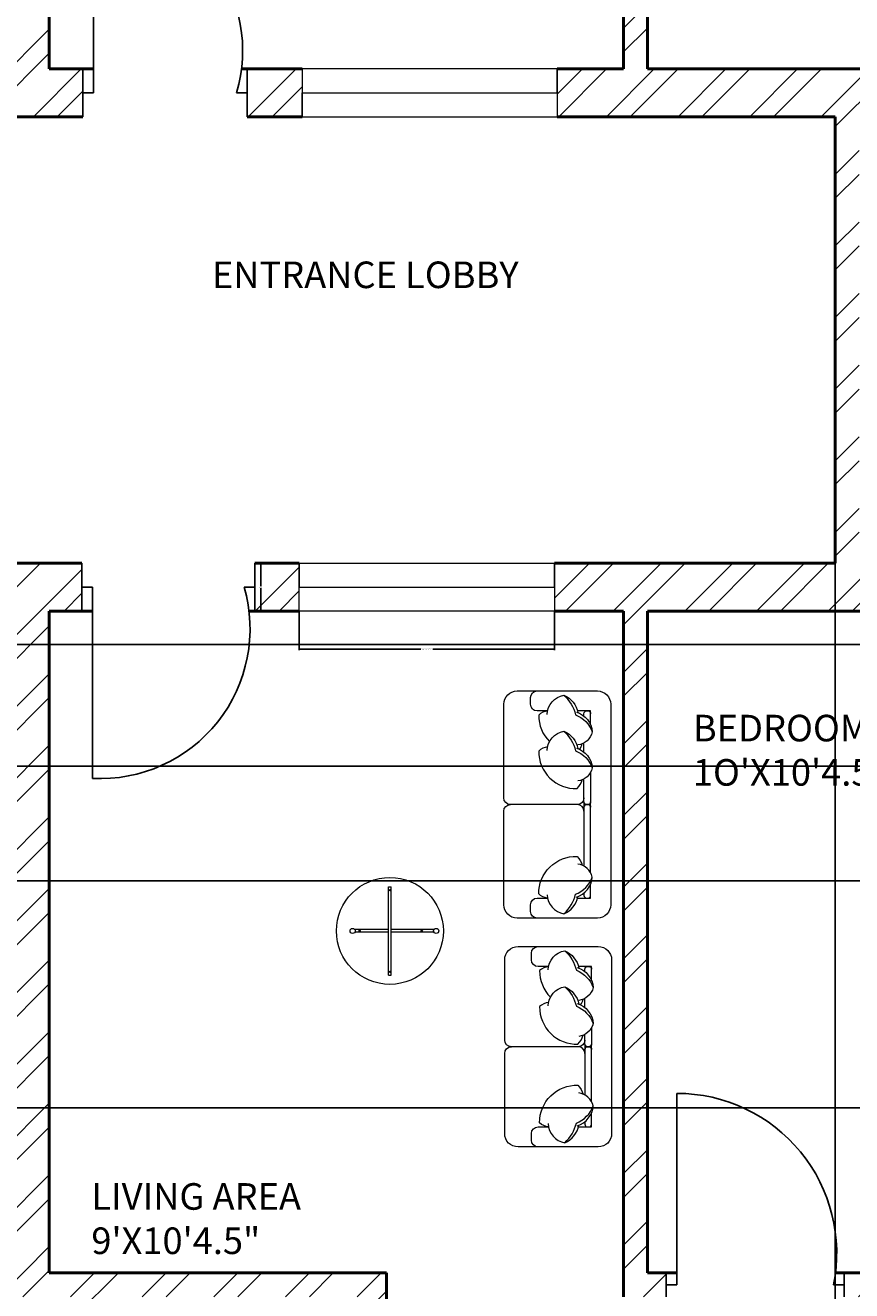
# Model space of a CAD drawing. Units: inches. Extents: x 1980 to 2738, y 1471 to 2568.
# Tile 14 of 22: x 2363 to 2519, y 1874 to 2112. Entities that reach past the tile are written whole.
import ezdxf

# ---------------------------------------------------------------- set-up
doc = ezdxf.new("R2010")
doc.units = ezdxf.units.IN
for name, color, linetype, lineweight in [('A-ANNO-DIMS', 2, 'Continuous', 18), ('A-AREA-IDEN', 7, 'Continuous', 18), ('A-DOOR', 31, 'Continuous', 25), ('A-FURN', 8, 'Continuous', 18), ('A-GLAZ', 141, 'Continuous', 18), ('A-WALL', 7, 'Continuous', 50)]:
    doc.layers.add(name, color=color, linetype=linetype, lineweight=lineweight)
doc.layers.add('A-WALL-PATT', color=9, linetype='Continuous', lineweight=13, true_color=0xd19cc7)
doc.styles.get("Standard").update_dxf_attribs({"font": 'arial.ttf'})
doc.dimstyles.get("Standard").update_dxf_attribs({"dimtxt": 0.18, "dimasz": 0.18, "dimexe": 0.18, "dimexo": 0.0625, "dimgap": 0.09, "dimtad": 0, "dimtih": 1, "dimtoh": 1, "dimdec": 4, "dimzin": 0, "dimdsep": 46, "dimtxsty": 'Standard', "dimcen": 0.09, "dimadec": 0, "dimazin": 0, "dimtfac": 1, "dimtdec": 4, "dimtofl": 0, "dimtmove": 0, "dimatfit": 3, "dimfxl": 1, "dimtolj": 1, "dimtzin": 0, "dimarcsym": 0})

# ---------------------------------------------------------------- blocks, each defined once
blk = doc.blocks.new('table r 343')
at = {"color": 0}
for p, q in [((-10, 10), (-10, 262.1)), ((10, 10), (10, 262.1)), ((-330.3, 10), (330.3, 10)), ((-330.3, 10), (-330.3, -10)), ((330.3, 10), (330.3, -10)), ((-330.3, -10), (330.3, -10)), ((-10, -330.3), (-10, -10)), ((10, -330.3), (10, -10))]:
    blk.add_line(p, q, dxfattribs=at)
for centre, radius in [((0, 0), 400), ((0, 278.7), 19.4), ((0, 226.8), 5), ((-306.1, 0), 5), ((306.1, 0), 5), ((0, -238.1), 5), ((0, -346.9), 19.4)]:
    blk.add_circle(centre, radius, dxfattribs=at)
blk = doc.blocks.new('WIN-48IN-WALL')
for p, q in [((0, 4.5), (0, 9)), ((0, 9), (0, 0)), ((48, 9), (0, 9)), ((48, 0), (48, 9)), ((48, 9), (48, 4.5)), ((48, 4.5), (0, 4.5)), ((0, 0), (48, 0))]:
    blk.add_line(p, q)
blk = doc.blocks.new('*D33')
at = {"layer": 'A-ANNO-DIMS', "color": 0, "lineweight": -2, "transparency": 16777216}
for p, q in [((2414.6, 2002.14), (2414.6, 1994.83)), ((2462.6, 2002.14), (2462.6, 1994.83)), ((2414.78, 1995.01), (2437.48, 1995.01)), ((2462.42, 1995.01), (2439.71, 1995.01))]:
    blk.add_line(p, q, dxfattribs=at)
at = {"layer": 'A-ANNO-DIMS', "color": 0, "transparency": 16777216}
for points in [[(2414.78, 1995.04), (2414.78, 1994.98), (2414.6, 1995.01)], [(2462.42, 1995.04), (2462.42, 1994.98), (2462.6, 1995.01)]]:
    blk.add_solid(points, dxfattribs=at)
at = {"layer": 'Defpoints', "color": 0, "transparency": 16777216}
for p in [(2414.6, 2002.21), (2462.6, 2002.21), (2414.6, 1995.01)]:
    blk.add_point(p, dxfattribs=at)
at = {"layer": 'A-ANNO-DIMS', "color": 0, "transparency": 16777216, "insert": (2438.6, 1995.01), "char_height": 0.18, "attachment_point": 5}
blk.add_mtext('\\A1;WINDOW 48 TYP.', dxfattribs=at)
blk = doc.blocks.new('*D34')
at = {"layer": 'A-ANNO-DIMS', "color": 0, "lineweight": -2, "transparency": 16777216}
for p, q in [((2414.53, 2011.21), (2407.22, 2011.21)), ((2407.4, 2011.03), (2407.4, 2006.89)), ((2407.4, 2002.39), (2407.4, 2006.52)), ((2414.53, 2002.21), (2407.22, 2002.21))]:
    blk.add_line(p, q, dxfattribs=at)
at = {"layer": 'A-ANNO-DIMS', "color": 0, "transparency": 16777216}
for points in [[(2407.37, 2011.03), (2407.43, 2011.03), (2407.4, 2011.21)], [(2407.37, 2002.39), (2407.43, 2002.39), (2407.4, 2002.21)]]:
    blk.add_solid(points, dxfattribs=at)
at = {"layer": 'Defpoints', "color": 0, "transparency": 16777216}
for p in [(2407.4, 2011.21), (2414.6, 2011.21), (2414.6, 2002.21)]:
    blk.add_point(p, dxfattribs=at)
at = {"layer": 'A-ANNO-DIMS', "color": 0, "transparency": 16777216, "insert": (2407.4, 2006.71), "char_height": 0.18, "attachment_point": 5}
blk.add_mtext('\\A1;9 TYP.', dxfattribs=at)
blk = doc.blocks.new('*D41')
at = {"layer": 'A-ANNO-DIMS', "color": 0, "lineweight": -2, "transparency": 16777216}
for p, q in [((2298.65, 2095.14), (2298.65, 1533.71)), ((2515.4, 2095.14), (2515.4, 1533.71)), ((2298.83, 1533.89), (2406.56, 1533.89)), ((2515.22, 1533.89), (2407.49, 1533.89))]:
    blk.add_line(p, q, dxfattribs=at)
at = {"layer": 'A-ANNO-DIMS', "color": 0, "transparency": 16777216}
for points in [[(2298.83, 1533.92), (2298.83, 1533.86), (2298.65, 1533.89)], [(2515.22, 1533.92), (2515.22, 1533.86), (2515.4, 1533.89)]]:
    blk.add_solid(points, dxfattribs=at)
at = {"layer": 'Defpoints', "color": 0, "transparency": 16777216}
for p in [(2298.65, 2095.21), (2515.4, 2095.21), (2515.4, 1533.89)]:
    blk.add_point(p, dxfattribs=at)
at = {"layer": 'A-ANNO-DIMS', "color": 0, "transparency": 16777216, "insert": (2407.03, 1533.89), "char_height": 0.18, "attachment_point": 5}
blk.add_mtext('\\A1;216.75', dxfattribs=at)
blk = doc.blocks.new('*D55')
at = {"layer": 'A-ANNO-DIMS', "color": 0, "lineweight": -2, "transparency": 16777216}
for p, q in [((2269.76, 1951.46), (2689.91, 1951.46)), ((2689.73, 1951.28), (2689.73, 1930.28)), ((2689.73, 1908.91), (2689.73, 1929.91)), ((2269.76, 1908.73), (2689.91, 1908.73))]:
    blk.add_line(p, q, dxfattribs=at)
at = {"layer": 'A-ANNO-DIMS', "color": 0, "transparency": 16777216}
for points in [[(2689.7, 1951.28), (2689.76, 1951.28), (2689.73, 1951.46)], [(2689.7, 1908.91), (2689.76, 1908.91), (2689.73, 1908.73)]]:
    blk.add_solid(points, dxfattribs=at)
at = {"layer": 'Defpoints', "color": 0, "transparency": 16777216}
for p in [(2269.7, 1951.46), (2689.73, 1951.46), (2269.7, 1908.73)]:
    blk.add_point(p, dxfattribs=at)
at = {"layer": 'A-ANNO-DIMS', "color": 0, "transparency": 16777216, "insert": (2689.73, 1930.09), "char_height": 0.18, "attachment_point": 5}
blk.add_mtext('\\A1;42.735', dxfattribs=at)
blk = doc.blocks.new('*D56')
at = {"layer": 'A-ANNO-DIMS', "color": 0, "lineweight": -2, "transparency": 16777216}
for p, q in [((2114.15, 1995.93), (2689.91, 1995.93)), ((2689.73, 1995.75), (2689.73, 1984.65)), ((2689.73, 1973.18), (2689.73, 1984.28)), ((2114.15, 1973), (2689.91, 1973))]:
    blk.add_line(p, q, dxfattribs=at)
at = {"layer": 'A-ANNO-DIMS', "color": 0, "transparency": 16777216}
for points in [[(2689.7, 1995.75), (2689.76, 1995.75), (2689.73, 1995.93)], [(2689.7, 1973.18), (2689.76, 1973.18), (2689.73, 1973)]]:
    blk.add_solid(points, dxfattribs=at)
at = {"layer": 'Defpoints', "color": 0, "transparency": 16777216}
for p in [(2114.08, 1995.93), (2689.73, 1995.93), (2114.08, 1973)]:
    blk.add_point(p, dxfattribs=at)
at = {"layer": 'A-ANNO-DIMS', "color": 0, "transparency": 16777216, "insert": (2689.73, 1984.47), "char_height": 0.18, "attachment_point": 5}
blk.add_mtext('\\A1;22.935', dxfattribs=at)

msp = doc.modelspace()

# ---------------------------------------------------------------- hatches: boundary and pattern name
at = {"layer": 'A-WALL-PATT'}
h = msp.add_hatch(dxfattribs=at)
h.set_pattern_fill('ANSI32', color=256)
h.paths.add_polyline_path([(2257.5661, 2416.2064), (2257.5661, 2420.7064), (2250.5833, 2420.7064), (2250.5833, 2462.7064), (2246.0833, 2462.7064), (2246.0833, 2420.7064), (2237.0791, 2420.7064), (2237.0791, 2411.7064), (2246.0833, 2411.7064), (2246.0833, 2291.7064), (2242.6109, 2291.7064), (2242.6109, 2287.2064), (2246.0833, 2287.2064), (2250.5833, 2287.2064), (2250.5833, 2291.7064), (2250.5833, 2411.7064), (2257.5661, 2411.7064)])
h.paths.add_polyline_path([(2387.0396, 2416.2064), (2387.0396, 2420.7064), (2367.5833, 2420.7064), (2367.5833, 2462.7064), (2358.5833, 2462.7064), (2358.5833, 2420.7064), (2329.3087, 2420.7064), (2329.3087, 2411.7064), (2358.5833, 2411.7064), (2358.5833, 2321.7275), (2358.5833, 2309.7064), (2347.3089, 2309.7064), (2293.3089, 2309.7064), (2293.3089, 2259.0771), (2297.8089, 2259.0771), (2297.8089, 2305.2064), (2347.3089, 2305.2064), (2347.3089, 2284.7412), (2351.8089, 2284.7412), (2351.8089, 2305.2064), (2372.3188, 2305.2064), (2372.3761, 2284.3899), (2377.0295, 2284.3899), (2377.0295, 2299.3058), (2377.0295, 2305.2064), (2426.5295, 2305.2064), (2426.5295, 2257.5573), (2431.0295, 2257.5573), (2431.0295, 2309.7064), (2377.0295, 2309.7064), (2367.5833, 2309.7064), (2367.5833, 2321.7275), (2367.5833, 2411.7064), (2387.0396, 2411.7064)])
h.paths.add_polyline_path([(2448.5267, 2416.2064), (2448.5267, 2420.7064), (2423.0396, 2420.7064), (2423.0396, 2411.7064), (2448.5267, 2411.7064)])
h.paths.add_polyline_path([(2130.9128, 2416.2064), (2130.9128, 2420.7064), (2105.0833, 2420.7064), (2105.0833, 2386.6942), (2114.0833, 2386.6942), (2114.0833, 2411.7064), (2130.9128, 2411.7064)])
h.paths.add_polyline_path([(2212.9478, 2420.7064), (2190.9128, 2420.7064), (2190.9128, 2411.7064), (2212.9478, 2411.7064), (2212.9478, 2416.2064)])
h.paths.add_polyline_path([(2114.0833, 2326.6942), (2105.0833, 2326.6942), (2105.0833, 2291.7064), (2081.0833, 2291.7064), (2081.0833, 2287.2064), (2105.0833, 2287.2064), (2105.0833, 2276.1935), (2114.0833, 2276.1935), (2114.0833, 2287.2064), (2166.3825, 2287.2064), (2166.3825, 2289.4564), (2166.3825, 2291.7064), (2114.0833, 2291.7064)])
h.paths.add_polyline_path([(2114.0833, 2252.1935), (2105.0833, 2252.1935), (2105.0833, 2233.2064), (2081.0833, 2233.2064), (2081.0833, 2228.7064), (2105.0833, 2228.7064), (2105.0833, 2213.4478), (2114.0833, 2213.4478), (2114.0833, 2228.7064), (2195.0833, 2228.7064), (2199.5833, 2228.7064), (2208.4455, 2228.7064), (2208.4455, 2230.9564), (2208.4455, 2233.2064), (2199.5833, 2233.2064), (2199.5833, 2287.2064), (2206.8904, 2287.2064), (2206.8904, 2289.4564), (2206.8904, 2291.7064), (2189.446, 2291.7064), (2189.446, 2289.4564), (2189.446, 2287.2064), (2195.0833, 2287.2064), (2195.0833, 2233.2064), (2114.0833, 2233.2064)])
h.paths.add_polyline_path([(2114.0833, 2153.4478), (2109.5833, 2153.4478), (2105.0833, 2153.4478), (2105.0833, 2135.2374), (2114.0833, 2135.2374)], flags=17)
h.paths.add_polyline_path([(2135.9619, 2095.4081), (2140.1805, 2095.4081), (2140.1805, 2104.2064), (2114.0833, 2104.2064), (2114.0833, 2110.3997), (2109.5833, 2110.3997), (2105.0833, 2110.3997), (2105.0833, 2104.2064), (2081.0833, 2104.2064), (2081.0833, 2099.7064), (2105.0833, 2099.7064), (2127.5416, 2099.8532), (2127.5416, 2056.9393), (2136.2133, 2056.9393)], flags=17)
h.paths.add_polyline_path([(2255.4895, 2104.2064), (2250.5833, 2104.2064), (2250.5833, 2233.2064), (2246.0833, 2233.2064), (2242.4941, 2233.2064), (2242.4941, 2228.7064), (2246.0833, 2228.7064), (2246.0833, 2104.2064), (2163.6825, 2104.2064), (2163.6825, 2099.8072), (2163.6825, 2095.4081), (2191.4325, 2095.4081), (2191.4325, 2011.2064), (2186.0833, 2011.2064), (2136.5143, 2010.8824), (2136.3702, 2032.9403), (2131.9559, 2032.9115), (2127.5416, 2032.8826), (2127.5416, 2006.7064), (2105.0833, 2006.7064), (2081.0833, 2006.7064), (2081.0833, 2002.2064), (2105.0833, 2002.2064), (2105.0833, 1995.9329), (2114.0833, 1995.9329), (2114.0833, 2002.2064), (2246.0833, 2002.2064), (2246.0833, 1877.7064), (2242.1358, 1877.7064), (2242.1358, 1873.2064), (2250.5833, 1873.2064), (2250.5833, 2002.2064), (2255.3335, 2002.2064), (2255.3335, 2011.2064), (2195.9325, 2011.2064), (2195.9325, 2095.2064), (2255.4895, 2095.2064), (2255.4895, 2099.5471)])
h.paths.add_polyline_path([(2199.5833, 1873.2064), (2209.827, 1873.2064), (2209.827, 1875.4564), (2209.827, 1877.7064), (2114.0833, 1877.7064), (2114.0833, 1890.0968), (2105.0833, 1890.0968), (2105.0833, 1877.7064), (2081.0833, 1877.7064), (2081.0833, 1873.2064), (2105.0833, 1873.2064), (2105.0833, 1857.7279), (2114.0833, 1857.7279), (2114.0833, 1873.2064), (2195.0833, 1873.2064), (2195.0833, 1819.2064), (2190.298, 1819.2064), (2190.298, 1814.7064), (2209.8976, 1814.7064), (2209.8976, 1816.9564), (2209.8976, 1819.2064), (2199.5833, 1819.2064)])
h.paths.add_polyline_path([(2114.0833, 1814.7064), (2166.2538, 1814.7064), (2166.2538, 1816.9564), (2166.2538, 1819.2064), (2114.0833, 1819.2064), (2114.0833, 1833.7279), (2109.5833, 1833.7279), (2105.0833, 1833.7279), (2105.0833, 1819.2064), (2081.0833, 1819.2064), (2081.0833, 1814.7064), (2105.0833, 1814.7064), (2105.0833, 1782.5516), (2114.0833, 1782.5516)])
h.paths.add_polyline_path([(2114.0833, 1722.5516), (2109.5833, 1722.5516), (2105.0833, 1722.5516), (2105.0833, 1685.7064), (2124.5104, 1685.7064), (2124.5104, 1690.2064), (2124.5104, 1694.7064), (2114.0833, 1694.7064)])
h.paths.add_polyline_path([(2218.8787, 1694.7064), (2184.5104, 1694.7064), (2184.5104, 1685.7064), (2218.8787, 1685.7064), (2218.8787, 1690.2064)])
h.paths.add_polyline_path([(2250.5833, 1819.2064), (2242.6431, 1819.2064), (2242.6431, 1816.9564), (2242.6431, 1814.7064), (2246.0833, 1814.7064), (2246.0833, 1694.7064), (2240.4035, 1694.7064), (2240.4035, 1690.2064), (2240.4035, 1685.7064), (2246.0833, 1685.7064), (2246.0833, 1643.7064), (2250.5833, 1643.7064), (2250.5833, 1685.7064), (2255.9859, 1685.7064), (2255.9859, 1690.2064), (2255.9859, 1694.7064), (2250.5833, 1694.7064)])
h.paths.add_polyline_path([(2297.4764, 1694.7064), (2279.3934, 1694.7064), (2279.3934, 1690.2064), (2279.3934, 1685.7064), (2297.4764, 1685.7064), (2297.4764, 1690.2064)])
h.paths.add_polyline_path([(2377.1596, 1694.7064), (2367.5833, 1694.7064), (2367.5833, 1787.7064), (2431.0295, 1787.7064), (2431.0295, 1792.2064), (2431.0295, 1849.4149), (2428.7795, 1849.4149), (2426.5295, 1849.4149), (2426.5295, 1792.2064), (2421.5833, 1792.2064), (2367.5833, 1792.2064), (2297.8089, 1792.2064), (2297.8089, 1850.2946), (2295.5589, 1850.2946), (2293.3089, 1850.2946), (2293.3089, 1792.2064), (2293.3089, 1787.7064), (2297.8089, 1787.7064), (2358.5833, 1787.7064), (2358.5833, 1694.7064), (2333.4764, 1694.7064), (2333.4764, 1685.7064), (2358.5833, 1685.7064), (2358.5833, 1643.7064), (2367.5833, 1643.7064), (2367.5833, 1685.7064), (2377.1596, 1685.7064)])
h.paths.add_polyline_path([(2442.4912, 1694.7064), (2413.1596, 1694.7064), (2413.1596, 1685.7064), (2442.4912, 1685.7064)])
h.paths.add_polyline_path([(2480.0833, 1814.7064), (2483.4816, 1814.7064), (2483.4816, 1817.9384), (2483.4816, 1819.2064), (2475.5833, 1819.2064), (2475.5833, 1694.7064), (2470.7283, 1694.7064), (2470.7283, 1685.7064), (2475.5833, 1685.7064), (2475.5833, 1643.7064), (2480.0833, 1643.7064), (2480.0833, 1685.7064), (2486.3293, 1685.7064), (2486.3293, 1690.2064), (2486.3293, 1694.7064), (2480.0833, 1694.7064)])
h.paths.add_polyline_path([(2621.0833, 1721.7349), (2612.0833, 1721.7349), (2612.0833, 1694.7064), (2586.1453, 1694.7064), (2586.1453, 1685.7064), (2621.0833, 1685.7064)])
h.paths.add_polyline_path([(2526.1453, 1690.2064), (2526.1453, 1694.7064), (2511.584, 1694.7064), (2511.584, 1690.2064), (2511.584, 1685.7064), (2526.1453, 1685.7064)])
h.paths.add_polyline_path([(2645.0833, 1819.2064), (2621.0833, 1819.2064), (2621.0833, 1835.8527), (2616.5833, 1835.8527), (2612.0833, 1835.8527), (2612.0833, 1819.2064), (2560.2541, 1819.2064), (2560.2541, 1814.7064), (2612.0833, 1814.7064), (2612.0833, 1781.7349), (2621.0833, 1781.7349), (2621.0833, 1814.7064), (2645.0833, 1814.7064)])
h.paths.add_polyline_path([(2645.0833, 1877.7064), (2621.0833, 1877.7064), (2621.0833, 1886.4375), (2612.0833, 1886.4375), (2612.0833, 1877.7064), (2517.1032, 1877.7064), (2517.1032, 1875.4564), (2517.1032, 1873.2064), (2526.5833, 1873.2064), (2526.5833, 1819.2064), (2516.6454, 1819.2064), (2516.6454, 1816.9564), (2516.6454, 1814.7064), (2536.4445, 1814.7064), (2536.4445, 1816.9564), (2536.4445, 1819.2064), (2531.0833, 1819.2064), (2531.0833, 1873.2064), (2612.0833, 1873.2064), (2612.0833, 1859.8527), (2621.0833, 1859.8527), (2621.0833, 1873.2064), (2645.0833, 1873.2064)])
h.paths.add_polyline_path([(2645.0833, 2006.7064), (2621.0833, 2006.7064), (2588.5085, 2006.7064), (2588.5085, 2052.9125), (2579.9045, 2052.9125), (2579.9045, 2011.2064), (2519.9045, 2011.2064), (2519.9045, 2095.2064), (2553.1204, 2095.2064), (2553.1204, 2104.2064), (2480.0833, 2104.2064), (2480.0833, 2228.7064), (2484.3832, 2228.7064), (2484.3832, 2230.9564), (2484.3832, 2233.2064), (2475.5833, 2233.2064), (2475.5833, 2104.2064), (2463.1308, 2104.2064), (2463.1308, 2095.2064), (2501.2463, 2095.2064), (2510.9045, 2095.2064), (2515.4045, 2095.2064), (2515.4045, 2011.2064), (2510.9045, 2011.2064), (2501.2463, 2011.2064), (2462.5957, 2011.2064), (2462.5957, 2002.2064), (2475.5833, 2002.2064), (2475.5833, 1873.2064), (2483.6146, 1873.2064), (2483.6146, 1875.4564), (2483.6146, 1877.7064), (2480.0833, 1877.7064), (2480.0833, 2002.2064), (2612.0833, 2002.2064), (2612.0833, 1996.309), (2621.0833, 1996.309), (2621.0833, 2002.2064), (2645.0833, 2002.2064)])
h.paths.add_polyline_path([(2588.5085, 2099.7277), (2621.0833, 2099.7277), (2645.0833, 2099.7064), (2645.0833, 2104.2064), (2621.0833, 2104.2064), (2621.0833, 2109.0038), (2616.5833, 2109.0038), (2612.0833, 2109.0038), (2612.0833, 2104.2064), (2575.0621, 2104.2064), (2575.0621, 2099.7064), (2575.0621, 2095.2064), (2579.9045, 2095.2064), (2579.9045, 2076.9125), (2588.5085, 2076.9125)], flags=17)
h.paths.add_polyline_path([(2367.5833, 2002.2064), (2373.7228, 2002.2064), (2373.7228, 2006.7064), (2373.7228, 2011.2064), (2350.7889, 2011.2064), (2350.7889, 2006.7064), (2350.7889, 2002.2064), (2358.5833, 2002.2064), (2358.5833, 1877.7064), (2293.3089, 1877.7064), (2293.3089, 1870.4987), (2297.8089, 1870.4987), (2297.8089, 1873.2064), (2347.3089, 1873.2064), (2347.3089, 1847.2208), (2351.8089, 1847.2208), (2351.8089, 1873.2064), (2372.5295, 1873.2064), (2372.5295, 1847.8619), (2377.0295, 1847.8619), (2377.0295, 1873.2064), (2426.5295, 1873.2064), (2426.5295, 1868.7339), (2431.0295, 1868.7339), (2431.0295, 1877.7064), (2367.5833, 1877.7064)])
h.paths.add_polyline_path([(2531.0833, 2287.2064), (2534.2285, 2287.2064), (2534.2285, 2291.7064), (2516.7886, 2291.7064), (2516.7886, 2287.2064), (2526.5833, 2287.2064), (2526.5833, 2233.2064), (2517.9112, 2233.2064), (2517.9112, 2230.9564), (2517.9112, 2228.7064), (2526.5833, 2228.7064), (2531.0833, 2228.7064), (2612.0833, 2228.7064), (2612.0833, 2206.8504), (2621.0833, 2206.8504), (2621.0833, 2228.7064), (2645.0833, 2228.7064), (2645.0833, 2233.2064), (2621.0833, 2233.2064), (2621.0833, 2241.8536), (2616.5833, 2241.8536), (2612.0833, 2241.8536), (2612.0833, 2233.2064), (2531.0833, 2233.2064)])
h.paths.add_polyline_path([(2645.0833, 2291.7064), (2621.0833, 2291.7064), (2621.0833, 2323.0138), (2616.5833, 2323.0138), (2612.0833, 2323.0138), (2612.0833, 2291.7064), (2559.6852, 2291.7064), (2559.6852, 2289.4564), (2559.6852, 2287.2064), (2612.0833, 2287.2064), (2612.0833, 2265.8536), (2621.0833, 2265.8536), (2621.0833, 2287.2064), (2645.0833, 2287.2064)])
h.paths.add_polyline_path([(2621.0833, 2420.7064), (2582.8189, 2420.7064), (2582.8189, 2411.7064), (2612.0833, 2411.7064), (2612.0833, 2383.0138), (2621.0833, 2383.0138)])
h.paths.add_polyline_path([(2480.0833, 2411.7064), (2485.7342, 2411.7064), (2485.7342, 2416.2064), (2485.7342, 2420.7064), (2480.0833, 2420.7064), (2480.0833, 2462.7064), (2475.5833, 2462.7064), (2475.5833, 2420.7064), (2469.4083, 2420.7064), (2469.4083, 2411.7064), (2475.5833, 2411.7064), (2475.5833, 2291.7064), (2475.5833, 2287.2064), (2482.9195, 2287.2064), (2482.9195, 2289.4564), (2482.9195, 2291.7064), (2480.0833, 2291.7064)])
h.paths.add_polyline_path([(2367.5833, 2228.7064), (2431.0295, 2228.7064), (2431.0295, 2233.2064), (2431.0295, 2237.4203), (2428.7795, 2237.4203), (2426.5295, 2237.4203), (2426.5295, 2233.2064), (2377.0295, 2233.2064), (2377.0295, 2260.3837), (2372.4423, 2260.3837), (2372.517, 2233.2635), (2351.8089, 2233.2064), (2351.8089, 2260.7412), (2347.3089, 2260.7412), (2347.3089, 2233.2064), (2297.8089, 2233.2064), (2297.8089, 2236.9324), (2293.3089, 2236.9324), (2293.3089, 2228.7064), (2358.5833, 2228.7064), (2358.5833, 2104.2064), (2353.3665, 2104.2064), (2353.3665, 2095.2064), (2373.8869, 2095.2064), (2373.8869, 2099.7064), (2373.8869, 2104.2064), (2367.5833, 2104.2064)])
h.paths.add_polyline_path([(2321.2323, 2104.2064), (2303.4895, 2104.2064), (2303.4895, 2095.2064), (2321.2323, 2095.2064), (2321.2323, 2099.7064)], flags=0)
h.paths.add_polyline_path([(2415.1308, 2099.7064), (2415.1308, 2104.2064), (2404.81, 2104.2064), (2404.81, 2095.2064), (2415.1308, 2095.2064)], flags=17)
h.paths.add_polyline_path([(2318.6336, 2011.2064), (2303.3335, 2011.2064), (2303.3335, 2002.2064), (2318.6336, 2002.2064)], flags=0)
h.paths.add_polyline_path([(2414.5957, 2011.2064), (2406.2461, 2011.2064), (2406.2461, 2006.7064), (2406.2461, 2002.2064), (2414.5957, 2002.2064)], flags=17)

# ---------------------------------------------------------------- linework, layer by layer
at = {"layer": 'A-DOOR'}
for p, q in [((2375.8869, 2099.7064), (2375.8869, 2135.7064)), ((2373.8869, 2104.2064), (2373.8869, 2095.2064)), ((2404.81, 2104.2064), (2404.81, 2095.2064)), ((2373.8869, 2095.2064), (2373.8869, 2099.7064)), ((2373.8869, 2099.7064), (2375.8869, 2099.7064)), ((2404.81, 2099.7064), (2402.81, 2099.7064)), ((2404.81, 2095.2064), (2404.81, 2099.7064)), ((2373.7228, 2011.2064), (2373.7228, 2002.2064)), ((2406.2461, 2002.2064), (2406.2461, 2011.2064)), ((2406.2461, 2011.2064), (2406.2461, 2006.7064)), ((2373.7228, 2002.2064), (2373.7228, 2006.7064)), ((2373.7228, 2006.7064), (2375.7228, 2006.7064)), ((2375.7228, 2006.7064), (2375.7228, 1970.7064)), ((2406.2461, 2006.7064), (2404.2461, 2006.7064)), ((2485.6146, 1875.4564), (2485.6146, 1911.4564)), ((2483.6146, 1877.7064), (2483.6146, 1873.2064)), ((2517.1032, 1873.2064), (2517.1032, 1877.7064)), ((2517.1032, 1877.7064), (2517.1032, 1875.4564)), ((2483.6146, 1873.2064), (2483.6146, 1875.4564)), ((2483.6146, 1875.4564), (2485.6146, 1875.4564)), ((2517.1032, 1875.4564), (2515.1032, 1875.4564))]:
    msp.add_line(p, q, dxfattribs=at)
for centre, radius, start, end in [((2375.8869, 2107.639), 28.0674, 343.583066, 90), ((2377.1618, 1998.866), 28.1963, 267.074603, 16.144742), ((2485.6146, 1881.3789), 30.0775, 348.64388, 90)]:
    msp.add_arc(centre, radius, start, end, dxfattribs=at)
at = {"layer": 'A-FURN', "ltscale": 0.03}
for points in [[(2453.0723, 1964.5406, -0.41421356), (2454.3292, 1965.7976, -0.41421356), (2453.0723, 1967.0545), (2453.0723, 1984.6513, -0.41421356), (2455.5862, 1987.1651), (2470.6692, 1987.1651, -0.41421356), (2473.183, 1984.6513), (2473.183, 1946.9438, -0.41421356), (2470.6692, 1944.43), (2455.5862, 1944.43, -0.41421356), (2453.0723, 1946.9438), (2453.0723, 1964.5406, -0.41421356), (2454.3292, 1965.7976, -0.41421356), (2453.0723, 1967.0545)], [(2453.2412, 1918.9767, -0.41421356), (2454.4981, 1920.2337, -0.41421356), (2453.2412, 1921.4906), (2453.2412, 1936.5736, -0.41421356), (2455.755, 1939.0874), (2470.838, 1939.0874, -0.41421356), (2473.3519, 1936.5736), (2473.3519, 1903.8937, -0.41421356), (2470.838, 1901.3799), (2455.755, 1901.3799, -0.41421356), (2453.2412, 1903.8937), (2453.2412, 1918.9767, -0.41421356), (2454.4981, 1920.2337, -0.41421356), (2453.2412, 1921.4906)]]:
    msp.add_lwpolyline(points, format="xyb", dxfattribs=at)
at = {"layer": 'A-FURN'}
for points in [[(2461.3043, 1983.3944), (2459.3569, 1983.3944, -0.41421356), (2458.1, 1984.6513), (2458.1, 1985.9082, -0.41421356), (2459.3569, 1987.1651)], [(2461.2283, 1982.7636, -0.35677236), (2464.3965, 1986.3652, -0.24954205), (2467.0073, 1983.1018, 9.61688035)], [(2464.3965, 1986.3652, -0.14772988), (2466.5566, 1982.6916, -0.21334276), (2469.7248, 1979.4502, -0.17866181)], [(2461.3049, 1983.3971, 0.16554063), (2459.6442, 1982.6196, 0.20023115), (2461.6668, 1977.6301, 0.12152332)], [(2466.7288, 1983.1991, -0.30666349), (2469.7248, 1979.4502, -0.30632997), (2466.9886, 1977.0011, 0.87284716)], [(2469.4122, 1980.7502), (2469.4122, 1983.3944), (2466.9421, 1983.3944, -0.41421356)], [(2468.1553, 1982.4352), (2468.1553, 1982.8916, -0.41421356), (2468.6581, 1983.3944), (2468.9095, 1983.3944, -0.41421356), (2469.4122, 1982.8916)], [(2461.2283, 1975.9927, -0.35677236), (2464.3965, 1979.5942, -0.24954205), (2467.0073, 1976.3309, 9.61688035)], [(2464.3965, 1979.5942, -0.14772988), (2466.5566, 1975.9206, -0.21334276), (2469.7248, 1972.6792, -0.17866181)], [(2461.3049, 1976.6262, 0.16554063), (2459.6442, 1975.8486, 0.42598917), (2466.8446, 1968.7895, 0.12152332), (2467.8371, 1970.4652, -7.11546429)], [(2466.7288, 1976.4281, -0.30666349), (2469.7248, 1972.6792, -0.30632997), (2466.9886, 1970.2301, 0.87284716)], [(2467.3457, 1976.1824, 0.07186538), (2467.8371, 1977.2362, -7.11546429)], [(2468.1553, 1975.6643), (2468.1553, 1977.3935, -0.41421356)], [(2469.4122, 1971.8882), (2469.4122, 1966.3003, -0.41421356), (2468.9095, 1965.7976), (2468.6581, 1965.7976, -0.41421356), (2468.1553, 1966.3003), (2468.1553, 1970.6225, -0.41421356)], [(2468.1553, 1967.0545, -0.41421356), (2466.8984, 1965.7976), (2454.3292, 1965.7976, -0.41421356)], [(2468.1553, 1967.0545, -0.41421356), (2466.8984, 1965.7976)], [(2468.1553, 1964.5406, 0.41421356), (2466.8984, 1965.7976), (2454.3292, 1965.7976, 0.41421356)], [(2468.1553, 1964.5406, 0.41421356), (2466.8984, 1965.7976)], [(2469.4122, 1952.936), (2469.4122, 1965.2948, 0.41421356), (2468.9095, 1965.7976), (2468.6581, 1965.7976, 0.41421356), (2468.1553, 1965.2948), (2468.1553, 1954.2016, 0.41421356)], [(2461.3049, 1948.198, -0.16554063), (2459.6442, 1948.9755, -0.42598917), (2466.8446, 1956.0346, -0.12152332), (2467.8371, 1954.3589, 7.11546429)], [(2466.7288, 1948.396, 0.30666349), (2469.7248, 1952.1449, 0.30632997), (2466.9886, 1954.594, -0.87284716)], [(2464.3965, 1945.2299, 0.14772988), (2466.5566, 1948.9035, 0.21334276), (2469.7248, 1952.1449, 0.17866181)], [(2459.3569, 1944.43, -0.41421356), (2458.1, 1945.6869), (2458.1, 1946.9438, -0.41421356), (2459.3569, 1948.2007), (2461.3043, 1948.2007)], [(2461.2283, 1948.8315, 0.35677236), (2464.3965, 1945.2299, 0.24954205), (2467.0073, 1948.4933, -9.61688035)], [(2468.1553, 1949.1599), (2468.1553, 1948.7035, 0.41421356), (2468.6581, 1948.2007), (2468.9095, 1948.2007, 0.41421356), (2469.4122, 1948.7035)], [(2461.4732, 1935.3167), (2459.5258, 1935.3167, -0.41421356), (2458.2689, 1936.5736), (2458.2689, 1937.8305, -0.41421356), (2459.5258, 1939.0874)], [(2461.3971, 1934.6859, -0.35677236), (2464.5653, 1938.2875, -0.24954205), (2467.1762, 1935.0241, 9.61688035)], [(2464.5653, 1938.2875, -0.14772988), (2466.7255, 1934.6139, -0.21334276), (2469.8937, 1931.3724, -0.17866181)], [(2461.4738, 1935.3194, 0.16554063), (2459.813, 1934.5418, 0.20023115), (2461.8356, 1929.5523, 0.12152332)], [(2466.8976, 1935.1214, -0.30666349), (2469.8937, 1931.3724, -0.30632997), (2467.1575, 1928.9234, 0.87284716)], [(2469.5811, 1932.6725), (2469.5811, 1935.3167), (2467.111, 1935.3167, -0.41421356)], [(2468.3242, 1934.3575), (2468.3242, 1934.8139, -0.41421356), (2468.827, 1935.3167), (2469.0783, 1935.3167, -0.41421356), (2469.5811, 1934.8139)], [(2461.3971, 1927.9149, -0.35677236), (2464.5653, 1931.5165, -0.24954205), (2467.1762, 1928.2531, 9.61688035)], [(2464.5653, 1931.5165, -0.14772988), (2466.7255, 1927.8429, -0.21334276), (2469.8937, 1924.6015, -0.17866181)], [(2461.4738, 1928.5484, 0.16554063), (2459.813, 1927.7709, 0.42598917), (2467.0135, 1920.7118, 0.12152332), (2468.0059, 1922.3875, -7.11546429)], [(2467.5145, 1928.1047, 0.07186538), (2468.0059, 1929.1584, -7.11546429)], [(2468.3242, 1927.5865), (2468.3242, 1929.3158, -0.41421356)], [(2466.8976, 1928.3504, -0.30666349), (2469.8937, 1924.6015, -0.30632997), (2467.1575, 1922.1524, 0.87284716)], [(2469.5811, 1923.8104), (2469.5811, 1920.7364, -0.41421356), (2469.0783, 1920.2337), (2468.827, 1920.2337, -0.41421356), (2468.3242, 1920.7364), (2468.3242, 1922.5448, -0.41421356)], [(2468.3242, 1921.4906, -0.41421356), (2467.0673, 1920.2337), (2454.4981, 1920.2337, -0.41421356)], [(2468.3242, 1921.4906, -0.41421356), (2467.0673, 1920.2337)], [(2468.3242, 1918.9767, 0.41421356), (2467.0673, 1920.2337), (2454.4981, 1920.2337, 0.41421356)], [(2468.3242, 1918.9767, 0.41421356), (2467.0673, 1920.2337)], [(2469.5811, 1909.8859), (2469.5811, 1919.7309, 0.41421356), (2469.0783, 1920.2337), (2468.827, 1920.2337, 0.41421356), (2468.3242, 1919.7309), (2468.3242, 1911.1516, 0.41421356)], [(2461.4738, 1905.1479, -0.16554063), (2459.813, 1905.9255, -0.42598917), (2467.0135, 1912.9846, -0.12152332), (2468.0059, 1911.3089, 7.11546429)], [(2466.8976, 1905.3459, 0.30666349), (2469.8937, 1909.0949, 0.30632997), (2467.1575, 1911.5439, -0.87284716)], [(2464.5653, 1902.1798, 0.14772988), (2466.7255, 1905.8535, 0.21334276), (2469.8937, 1909.0949, 0.17866181)], [(2459.5258, 1901.3799, -0.41421356), (2458.2689, 1902.6368), (2458.2689, 1903.8937, -0.41421356), (2459.5258, 1905.1507), (2461.4732, 1905.1507)], [(2461.3971, 1905.7814, 0.35677236), (2464.5653, 1902.1798, 0.24954205), (2467.1762, 1905.4432, -9.61688035)], [(2468.3242, 1906.1098), (2468.3242, 1905.6534, 0.41421356), (2468.827, 1905.1507), (2469.0783, 1905.1507, 0.41421356), (2469.5811, 1905.6534)]]:
    msp.add_lwpolyline(points, format="xyb", dxfattribs=at)
for points in [[(2469.4122, 1965.2948), (2469.4122, 1966.3003, -0.41421356), (2468.9095, 1965.7976), (2468.6581, 1965.7976, -0.41421356), (2468.1553, 1966.3003), (2468.1553, 1965.2948, -0.41421356), (2468.6581, 1965.7976), (2468.9095, 1965.7976, -0.41421356)], [(2469.5811, 1919.7309), (2469.5811, 1920.7364, -0.41421356), (2469.0783, 1920.2337), (2468.827, 1920.2337, -0.41421356), (2468.3242, 1920.7364), (2468.3242, 1919.7309, -0.41421356), (2468.827, 1920.2337), (2469.0783, 1920.2337, -0.41421356)]]:
    msp.add_lwpolyline(points, format="xyb", close=True, dxfattribs=at)
for points in [[(2466.9421, 1948.2007), (2469.4122, 1948.2007), (2469.4122, 1950.8449)], [(2467.111, 1905.1507), (2469.5811, 1905.1507), (2469.5811, 1907.7949)]]:
    msp.add_lwpolyline(points, dxfattribs=at)
at = {"layer": 'A-GLAZ'}
for p, q in [((2415.1308, 2104.2064), (2415.1308, 2095.2064)), ((2463.1308, 2104.2064), (2415.1308, 2104.2064)), ((2463.1308, 2099.7064), (2463.1308, 2104.2064)), ((2463.1308, 2104.2064), (2463.1308, 2095.2064)), ((2415.1308, 2095.2064), (2415.1308, 2099.7064)), ((2415.1308, 2099.7064), (2439.1308, 2099.7064)), ((2439.1308, 2099.7064), (2463.1308, 2099.7064)), ((2415.1308, 2095.2064), (2463.1308, 2095.2064))]:
    msp.add_line(p, q, dxfattribs=at)
at = {"layer": 'A-WALL'}
for p, q in [((2475.5833, 2233.2064), (2475.5833, 2104.2064)), ((2367.5833, 2104.2064), (2367.5833, 2228.7064)), ((2480.0833, 2228.7064), (2480.0833, 2104.2064)), ((2367.5833, 2104.2064), (2375.8869, 2104.2064)), ((2403.7436, 2104.2064), (2415.1308, 2104.2064)), ((2463.1308, 2104.2064), (2475.5833, 2104.2064)), ((2480.0833, 2104.2064), (2553.1204, 2104.2064)), ((2373.8869, 2095.2064), (2353.3665, 2095.2064)), ((2415.1308, 2095.2064), (2404.81, 2095.2064)), ((2501.2463, 2095.2064), (2463.1308, 2095.2064)), ((2501.2463, 2095.2064), (2501.2463, 2095.2064)), ((2501.2463, 2095.2064), (2510.9045, 2095.2064)), ((2510.9045, 2095.2064), (2515.4045, 2095.2064)), ((2515.4045, 2095.2064), (2515.4045, 2011.2064)), ((2373.7228, 2011.2064), (2350.7889, 2011.2064)), ((2414.5957, 2011.2064), (2406.2461, 2011.2064)), ((2501.2463, 2011.2064), (2462.5957, 2011.2064)), ((2510.9045, 2011.2064), (2501.2463, 2011.2064)), ((2501.2463, 2011.2064), (2510.9045, 2011.2064)), ((2510.9045, 2011.2064), (2510.9045, 2011.2064)), ((2515.4045, 2011.2064), (2510.9045, 2011.2064)), ((2367.5833, 2002.2064), (2367.5833, 1877.7064)), ((2375.7228, 2002.2064), (2367.5833, 2002.2064)), ((2414.5957, 2002.2064), (2405.1595, 2002.2064)), ((2475.5833, 2002.2064), (2462.5957, 2002.2064)), ((2475.5833, 2002.2064), (2475.5833, 1873.2064)), ((2612.0833, 2002.2064), (2480.0833, 2002.2064)), ((2480.0833, 2002.2064), (2480.0833, 1877.7064)), ((2431.0295, 1877.7064), (2367.5833, 1877.7064)), ((2431.0295, 1877.7064), (2431.0295, 1868.7339)), ((2485.6146, 1877.7064), (2480.0833, 1877.7064)), ((2612.0833, 1877.7064), (2515.467, 1877.7064))]:
    msp.add_line(p, q, dxfattribs=at)

# ---------------------------------------------------------------- block references
at = {"layer": 'A-FURN', "xscale": 0.0251383443972704, "yscale": 0.0251383443972704, "zscale": 0.0251383443972704, "rotation": 89.99999999999999}
msp.add_blockref('table r 343', (2431.6494, 1942.0145), dxfattribs=at)
at = {"layer": 'A-GLAZ', "extrusion": (0, 0, -1), "zscale": -1}
msp.add_blockref('WIN-48IN-WALL', (-2462.5961, 2002.206), dxfattribs=at)

# ---------------------------------------------------------------- texts
at = {"layer": 'A-AREA-IDEN', "insert": (2398.1696, 2067.9574), "char_height": 5, "width": 71.988322, "attachment_point": 1}
msp.add_mtext('ENTRANCE LOBBY', dxfattribs=at)
at = {"layer": 'A-AREA-IDEN', "char_height": 5, "attachment_point": 1}
for s, width, insert in [('BEDROOM\\P1O\'X10\'4.5"', 105.31612, (2488.6336, 1982.6786)), ('LIVING AREA\\P9\'X10\'4.5"', 101.701555, (2375.507, 1894.5612))]:
    msp.add_mtext_dynamic_manual_height_columns(s, width=width, gutter_width=12.5, heights=[0], dxfattribs=dict(at, insert=insert))

# ---------------------------------------------------------------- dimensions: what is measured, and where the dimension line sits
at = {"layer": 'A-ANNO-DIMS'}
dim = msp.add_linear_dim(base=(2515.4045, 1533.8857), p1=(2298.6516, 2095.2064), p2=(2515.4045, 2095.2064), dimstyle='Standard', override={"dimdec": 2, "dimlfac": 1, "dimrnd": 0, "dimzin": 0, "dimdsep": 46, "dimlunit": 2}, dxfattribs=at)
dim.commit()
dim.dimension.update_dxf_attribs({"geometry": '*D41', "text_midpoint": (2407.0281, 1533.8857)})
for base, p1, p2, angle, text, picture, middle in [((2407.3957, 2011.2064), (2414.5957, 2002.2064), (2414.5957, 2011.2064), 90, '<> TYP.', '*D34', (2407.3957, 2006.7064)), ((2414.5957, 1995.0064), (2462.5957, 2002.2064), (2414.5957, 2002.2064), 180, 'WINDOW <> TYP.', '*D33', (2438.5957, 1995.0064))]:
    dim = msp.add_linear_dim(base=base, p1=p1, p2=p2, angle=angle, text=text, dimstyle='Standard', override={"dimdec": 0, "dimlfac": 1, "dimrnd": 0, "dimzin": 0, "dimdsep": 46, "dimlunit": 2}, dxfattribs=at)
    dim.commit()
    dim.dimension.update_dxf_attribs({"geometry": picture, "text_midpoint": middle})
for base, p1, p2, picture, middle in [((2689.7333, 1995.9329), (2114.0833, 1972.9983), (2114.0833, 1995.9329), '*D56', (2689.7333, 1984.4656)), ((2689.7333, 1951.461), (2269.6968, 1908.7258), (2269.6968, 1951.461), '*D55', (2689.7333, 1930.0934))]:
    dim = msp.add_linear_dim(base=base, p1=p1, p2=p2, angle=90, dimstyle='Standard', override={"dimdec": 3, "dimlfac": 1, "dimrnd": 0, "dimzin": 0, "dimdsep": 46, "dimlunit": 2}, dxfattribs=at)
    dim.commit()
    dim.dimension.update_dxf_attribs({"geometry": picture, "text_midpoint": middle})

doc.saveas('drawing.dxf')
